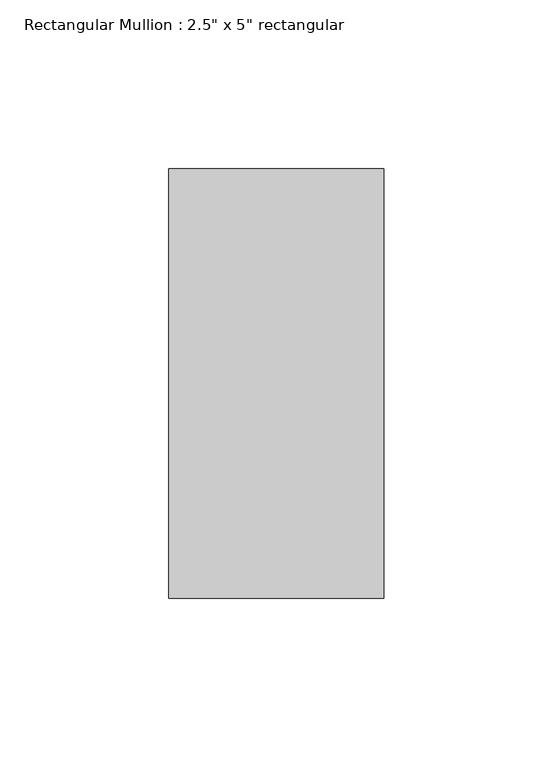
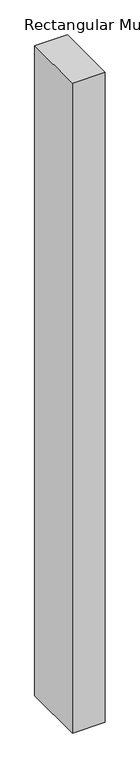
"""IFC4 building model written with IfcOpenShell, lengths in millimetres: member geometry."""

from ifc_helpers import new_model, si_unit, frame, origin, place, context, project, spatial, polyline, outline, extrude, source, transform, mapped, element, save


def member_f6f550b4(model_context):
    return source(origin(), model_context, "Body", "SweptSolid", [
        extrude(outline(polyline([(0.0, 63.5), (0.0, -63.5), (-63.5, -63.5), (-63.5, 63.5), (0.0, 63.5)])), frame((0.0, 0.0, -1337.1154286), z_axis=(0.0, 0.0, 1.0), x_axis=(1.0, 0.0, 0.0)), (0.0, 0.0, 1.0), 1337.1154286),
    ])


if __name__ == "__main__":
    model = new_model("IFC4")
    model_context = context("Model", 3, world=origin())
    ifc_project = project(units=[si_unit("LENGTHUNIT", "METRE", prefix="MILLI")], contexts=[model_context])
    site = spatial("IfcSite", under=ifc_project)
    building = spatial("IfcBuilding", under=site)
    placement = place(None, origin())
    member_shape = member_f6f550b4(model_context)
    element("IfcMember", 1, ObjectType="Rectangular Mullion : 2.5\" x 5\" rectangular", at=placement, inside=building, context=model_context, shape_type="MappedRepresentation", body=[
        mapped(member_shape, transform((0.0, 0.0, 0.0), x_axis=(1.0, 0.0, 0.0), y_axis=(0.0, 1.0, 0.0), z_axis=(0.0, 0.0, 1.0))),
    ])
    save(model, "model.ifc")

# Revit data of these elements
# Type "Rectangular Mullion : 2.5\" x 5\" rectangular"
#   built-in parameter 1007304 = 0.416667 (stored number, unit not read)
#   built-in parameter 1007301 = 0.104167 (stored number, unit not read)
#   built-in parameter 1007300 = 0.104167 (stored number, unit not read)
# Element 1 (IfcMember, "Rectangular Mullion : 2.5\" x 5\" rectangular")
#   Materials on its faces: "Iron, Ductile"
# Materials
#   "Iron, Ductile": class "Metal", colour RGB 0 0 0, transparency 0, Description = "Ductile cast iron", Cost = 0
